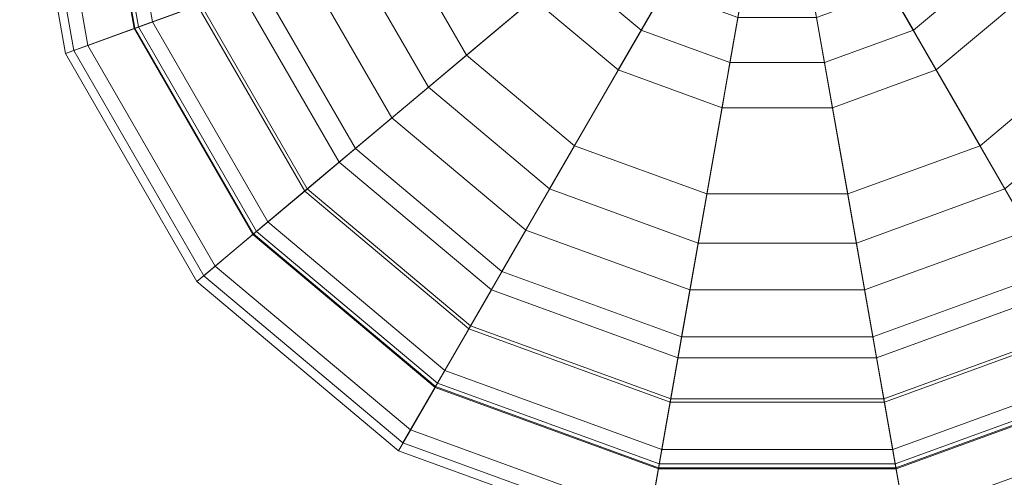
# Model space of a CAD drawing. Units: inches. Extents: x 375 to 1122, y 27 to 1069.
# Tile 41 of 155: x 717.909 to 719.669, y 297.867 to 298.684. Entities that reach past the tile are written whole.
import ezdxf

# ---------------------------------------------------------------- set-up
doc = ezdxf.new("R2010")
doc.units = ezdxf.units.IN
doc.layers.add('Furniture', color=30, linetype='Continuous', lineweight=18)

# ---------------------------------------------------------------- blocks, each defined once
blk = doc.blocks.new('A$C403C54AD')
for points in [[(1.191834, 0.889704, -0.031825), (1.180252, 0.857884, -0.028747), (1.180252, 0.857884, -0.028747), (1.180252, 0.891746, -0.031825)], [(1.202018, 0.883824, -0.031825), (1.180252, 0.857884, -0.028747), (1.180252, 0.857884, -0.028747), (1.191834, 0.889704, -0.031825)], [(1.209578, 0.874815, -0.031825), (1.180252, 0.857884, -0.028747), (1.180252, 0.857884, -0.028747), (1.202018, 0.883824, -0.031825)], [(1.192562, 0.864991, -0.02532), (1.206749, 0.873182, -0.028594), (1.199919, 0.881322, -0.028594), (1.189389, 0.868773, -0.02532)], [(1.193338, 0.873479, 0.061451), (1.186756, 0.865635, 0.054084), (1.183713, 0.867392, 0.054084), (1.187215, 0.877014, 0.061451)], [(1.195951, 0.866948, 0.063639), (1.201568, 0.87019, 0.073031), (1.196073, 0.876739, 0.073031), (1.191904, 0.87177, 0.063639)], [(1.2136, 0.863764, -0.031825), (1.180252, 0.857884, -0.028747), (1.180252, 0.857884, -0.028747), (1.209578, 0.874815, -0.031825)], [(1.185975, 0.864705, 0.057003), (1.191904, 0.87177, 0.063639), (1.186452, 0.874918, 0.063639), (1.183297, 0.866251, 0.057003)], [(1.210344, 0.86319, 0.131159), (1.213207, 0.863695, 0.117935), (1.209232, 0.874616, 0.117935), (1.206714, 0.873162, 0.131159)], [(1.210384, 0.863197, -0.028594), (1.2136, 0.863764, -0.031825), (1.209578, 0.874815, -0.031825), (1.206749, 0.873182, -0.028594)], [(1.213207, 0.863695, 0.117935), (1.212542, 0.863578, 0.089693), (1.208648, 0.874278, 0.089693), (1.209232, 0.874616, 0.117935)], [(1.212542, 0.863578, 0.089693), (1.207259, 0.862646, 0.071684), (1.204002, 0.871596, 0.071684), (1.208648, 0.874278, 0.089693)], [(1.197882, 0.868063, 0.061451), (1.189015, 0.862943, 0.054084), (1.186756, 0.865635, 0.054084), (1.193338, 0.873479, 0.061451)], [(1.19425, 0.860352, -0.02532), (1.210384, 0.863197, -0.028594), (1.206749, 0.873182, -0.028594), (1.192562, 0.864991, -0.02532)], [(1.204491, 0.862158, 0.073031), (1.209521, 0.863045, 0.090178), (1.205991, 0.872744, 0.090178), (1.201568, 0.87019, 0.073031)], [(1.205423, 0.862322, 0.140564), (1.210344, 0.86319, 0.131159), (1.206714, 0.873162, 0.131159), (1.202387, 0.870664, 0.140564)], [(1.210169, 0.863159, 0.117718), (1.207402, 0.862671, 0.130354), (1.204128, 0.871669, 0.130354), (1.206561, 0.873073, 0.117718)], [(1.209521, 0.863045, 0.090178), (1.210169, 0.863159, 0.117718), (1.206561, 0.873073, 0.117718), (1.205991, 0.872744, 0.090178)], [(1.187963, 0.862336, 0.057003), (1.195951, 0.866948, 0.063639), (1.191904, 0.87177, 0.063639), (1.185975, 0.864705, 0.057003)], [(1.207259, 0.862646, 0.071684), (1.2003, 0.861419, 0.061451), (1.197882, 0.868063, 0.061451), (1.204002, 0.871596, 0.071684)], [(1.207402, 0.862671, 0.130354), (1.202392, 0.861788, 0.140564), (1.199721, 0.869125, 0.140564), (1.204128, 0.871669, 0.130354)], [(1.202392, 0.861788, 0.140564), (1.205423, 0.862322, 0.140564), (1.202387, 0.870664, 0.140564), (1.199721, 0.869125, 0.140564)], [(1.198104, 0.861032, 0.063639), (1.204491, 0.862158, 0.073031), (1.201568, 0.87019, 0.073031), (1.195951, 0.866948, 0.063639)], [(1.190789, 0.863967, -0.022455), (1.192562, 0.864991, -0.02532), (1.189389, 0.868773, -0.02532), (1.188073, 0.867204, -0.022455)], [(1.2003, 0.861419, 0.061451), (1.190217, 0.859641, 0.054084), (1.189015, 0.862943, 0.054084), (1.197882, 0.868063, 0.061451)], [(1.187242, 0.861919, -0.020408), (1.190789, 0.863967, -0.022455), (1.188073, 0.867204, -0.022455), (1.18544, 0.864067, -0.020408)], [(1.189021, 0.85943, 0.057003), (1.198104, 0.861032, 0.063639), (1.195951, 0.866948, 0.063639), (1.187963, 0.862336, 0.057003)], [(1.192234, 0.859997, -0.022455), (1.19425, 0.860352, -0.02532), (1.192562, 0.864991, -0.02532), (1.190789, 0.863967, -0.022455)], [(1.1882, 0.859285, -0.020408), (1.192234, 0.859997, -0.022455), (1.190789, 0.863967, -0.022455), (1.187242, 0.861919, -0.020408)], [(1.2136, 0.852004, -0.031825), (1.180252, 0.857884, -0.028747), (1.180252, 0.857884, -0.028747), (1.2136, 0.863764, -0.031825)], [(1.212542, 0.85219, 0.089693), (1.207259, 0.853122, 0.071684), (1.207259, 0.862646, 0.071684), (1.212542, 0.863578, 0.089693)], [(1.210344, 0.852578, 0.131159), (1.213207, 0.852073, 0.117935), (1.213207, 0.863695, 0.117935), (1.210344, 0.86319, 0.131159)], [(1.210384, 0.852571, -0.028594), (1.2136, 0.852004, -0.031825), (1.2136, 0.863764, -0.031825), (1.210384, 0.863197, -0.028594)], [(1.19425, 0.855416, -0.02532), (1.210384, 0.852571, -0.028594), (1.210384, 0.863197, -0.028594), (1.19425, 0.860352, -0.02532)], [(1.205423, 0.853446, 0.140564), (1.210344, 0.852578, 0.131159), (1.210344, 0.86319, 0.131159), (1.205423, 0.862322, 0.140564)], [(1.210169, 0.852609, 0.117718), (1.207402, 0.853097, 0.130354), (1.207402, 0.862671, 0.130354), (1.210169, 0.863159, 0.117718)], [(1.209521, 0.852723, 0.090178), (1.210169, 0.852609, 0.117718), (1.210169, 0.863159, 0.117718), (1.209521, 0.863045, 0.090178)], [(1.207259, 0.853122, 0.071684), (1.2003, 0.854349, 0.061451), (1.2003, 0.861419, 0.061451), (1.207259, 0.862646, 0.071684)], [(1.207402, 0.853097, 0.130354), (1.202392, 0.85398, 0.140564), (1.202392, 0.861788, 0.140564), (1.207402, 0.862671, 0.130354)], [(1.204491, 0.85361, 0.073031), (1.209521, 0.852723, 0.090178), (1.209521, 0.863045, 0.090178), (1.204491, 0.862158, 0.073031)], [(1.202392, 0.85398, 0.140564), (1.205423, 0.853446, 0.140564), (1.205423, 0.862322, 0.140564), (1.202392, 0.861788, 0.140564)], [(1.198104, 0.854736, 0.063639), (1.204491, 0.85361, 0.073031), (1.204491, 0.862158, 0.073031), (1.198104, 0.861032, 0.063639)], [(1.2003, 0.854349, 0.061451), (1.190217, 0.856127, 0.054084), (1.190217, 0.859641, 0.054084), (1.2003, 0.861419, 0.061451)], [(1.189021, 0.856338, 0.057003), (1.198104, 0.854736, 0.063639), (1.198104, 0.861032, 0.063639), (1.189021, 0.85943, 0.057003)], [(1.1882, 0.856482, -0.020408), (1.192234, 0.855771, -0.022455), (1.192234, 0.859997, -0.022455), (1.1882, 0.859285, -0.020408)], [(1.192234, 0.855771, -0.022455), (1.19425, 0.855416, -0.02532), (1.19425, 0.860352, -0.02532), (1.192234, 0.859997, -0.022455)], [(1.209578, 0.840953, -0.031825), (1.180252, 0.857884, -0.028747), (1.180252, 0.857884, -0.028747), (1.2136, 0.852004, -0.031825)], [(1.202018, 0.831944, -0.031825), (1.180252, 0.857884, -0.028747), (1.180252, 0.857884, -0.028747), (1.209578, 0.840953, -0.031825)], [(1.191834, 0.826064, -0.031825), (1.180252, 0.857884, -0.028747), (1.180252, 0.857884, -0.028747), (1.202018, 0.831944, -0.031825)], [(1.180252, 0.824022, -0.031825), (1.180252, 0.857884, -0.028747), (1.180252, 0.857884, -0.028747), (1.191834, 0.826064, -0.031825)], [(1.187242, 0.853848, -0.020408), (1.190789, 0.851801, -0.022455), (1.192234, 0.855771, -0.022455), (1.1882, 0.856482, -0.020408)], [(1.187963, 0.853432, 0.057003), (1.195951, 0.84882, 0.063639), (1.198104, 0.854736, 0.063639), (1.189021, 0.856338, 0.057003)], [(1.197882, 0.847705, 0.061451), (1.189015, 0.852825, 0.054084), (1.190217, 0.856127, 0.054084), (1.2003, 0.854349, 0.061451)], [(1.190789, 0.851801, -0.022455), (1.192562, 0.850777, -0.02532), (1.19425, 0.855416, -0.02532), (1.192234, 0.855771, -0.022455)], [(1.192562, 0.850777, -0.02532), (1.206749, 0.842586, -0.028594), (1.210384, 0.852571, -0.028594), (1.19425, 0.855416, -0.02532)], [(1.195951, 0.84882, 0.063639), (1.201568, 0.845577, 0.073031), (1.204491, 0.85361, 0.073031), (1.198104, 0.854736, 0.063639)], [(1.204002, 0.844172, 0.071684), (1.197882, 0.847705, 0.061451), (1.2003, 0.854349, 0.061451), (1.207259, 0.853122, 0.071684)], [(1.18544, 0.851701, -0.020408), (1.188073, 0.848564, -0.022455), (1.190789, 0.851801, -0.022455), (1.187242, 0.853848, -0.020408)], [(1.199721, 0.846643, 0.140564), (1.202387, 0.845104, 0.140564), (1.205423, 0.853446, 0.140564), (1.202392, 0.85398, 0.140564)], [(1.204128, 0.844099, 0.130354), (1.199721, 0.846643, 0.140564), (1.202392, 0.85398, 0.140564), (1.207402, 0.853097, 0.130354)], [(1.185975, 0.851063, 0.057003), (1.191904, 0.843998, 0.063639), (1.195951, 0.84882, 0.063639), (1.187963, 0.853432, 0.057003)], [(1.201568, 0.845577, 0.073031), (1.205991, 0.843024, 0.090178), (1.209521, 0.852723, 0.090178), (1.204491, 0.85361, 0.073031)], [(1.202387, 0.845104, 0.140564), (1.206714, 0.842606, 0.131159), (1.210344, 0.852578, 0.131159), (1.205423, 0.853446, 0.140564)], [(1.208648, 0.84149, 0.089693), (1.204002, 0.844172, 0.071684), (1.207259, 0.853122, 0.071684), (1.212542, 0.85219, 0.089693)], [(1.206561, 0.842695, 0.117718), (1.204128, 0.844099, 0.130354), (1.207402, 0.853097, 0.130354), (1.210169, 0.852609, 0.117718)], [(1.193338, 0.842289, 0.061451), (1.186756, 0.850133, 0.054084), (1.189015, 0.852825, 0.054084), (1.197882, 0.847705, 0.061451)], [(1.205991, 0.843024, 0.090178), (1.206561, 0.842695, 0.117718), (1.210169, 0.852609, 0.117718), (1.209521, 0.852723, 0.090178)], [(1.206714, 0.842606, 0.131159), (1.209232, 0.841152, 0.117935), (1.213207, 0.852073, 0.117935), (1.210344, 0.852578, 0.131159)], [(1.206749, 0.842586, -0.028594), (1.209578, 0.840953, -0.031825), (1.2136, 0.852004, -0.031825), (1.210384, 0.852571, -0.028594)], [(1.209232, 0.841152, 0.117935), (1.208648, 0.84149, 0.089693), (1.212542, 0.85219, 0.089693), (1.213207, 0.852073, 0.117935)], [(1.188073, 0.848564, -0.022455), (1.189389, 0.846995, -0.02532), (1.192562, 0.850777, -0.02532), (1.190789, 0.851801, -0.022455)], [(1.183297, 0.849517, 0.057003), (1.186452, 0.84085, 0.063639), (1.191904, 0.843998, 0.063639), (1.185975, 0.851063, 0.057003)], [(1.189389, 0.846995, -0.02532), (1.199919, 0.834446, -0.028594), (1.206749, 0.842586, -0.028594), (1.192562, 0.850777, -0.02532)], [(1.187215, 0.838754, 0.061451), (1.183713, 0.848375, 0.054084), (1.186756, 0.850133, 0.054084), (1.193338, 0.842289, 0.061451)], [(1.191904, 0.843998, 0.063639), (1.196073, 0.839029, 0.073031), (1.201568, 0.845577, 0.073031), (1.195951, 0.84882, 0.063639)], [(1.19788, 0.836876, 0.071684), (1.193338, 0.842289, 0.061451), (1.197882, 0.847705, 0.061451), (1.204002, 0.844172, 0.071684)], [(1.185114, 0.844527, -0.02532), (1.190717, 0.829133, -0.028594), (1.199919, 0.834446, -0.028594), (1.189389, 0.846995, -0.02532)], [(1.194703, 0.840662, 0.140564), (1.196681, 0.838304, 0.140564), (1.202387, 0.845104, 0.140564), (1.199721, 0.846643, 0.140564)], [(1.197973, 0.836765, 0.130354), (1.194703, 0.840662, 0.140564), (1.199721, 0.846643, 0.140564), (1.204128, 0.844099, 0.130354)], [(1.196073, 0.839029, 0.073031), (1.199356, 0.835117, 0.090178), (1.205991, 0.843024, 0.090178), (1.201568, 0.845577, 0.073031)], [(1.196681, 0.838304, 0.140564), (1.199893, 0.834477, 0.131159), (1.206714, 0.842606, 0.131159), (1.202387, 0.845104, 0.140564)], [(1.180252, 0.84367, -0.02532), (1.180252, 0.827288, -0.028594), (1.190717, 0.829133, -0.028594), (1.185114, 0.844527, -0.02532)], [(1.201328, 0.832767, 0.089693), (1.19788, 0.836876, 0.071684), (1.204002, 0.844172, 0.071684), (1.208648, 0.84149, 0.089693)], [(1.186452, 0.84085, 0.063639), (1.18867, 0.834755, 0.073031), (1.196073, 0.839029, 0.073031), (1.191904, 0.843998, 0.063639)], [(1.199779, 0.834612, 0.117718), (1.197973, 0.836765, 0.130354), (1.204128, 0.844099, 0.130354), (1.206561, 0.842695, 0.117718)], [(1.199356, 0.835117, 0.090178), (1.199779, 0.834612, 0.117718), (1.206561, 0.842695, 0.117718), (1.205991, 0.843024, 0.090178)], [(1.199893, 0.834477, 0.131159), (1.201762, 0.83225, 0.117935), (1.209232, 0.841152, 0.117935), (1.206714, 0.842606, 0.131159)], [(1.199919, 0.834446, -0.028594), (1.202018, 0.831944, -0.031825), (1.209578, 0.840953, -0.031825), (1.206749, 0.842586, -0.028594)], [(1.189632, 0.832114, 0.071684), (1.187215, 0.838754, 0.061451), (1.193338, 0.842289, 0.061451), (1.19788, 0.836876, 0.071684)], [(1.201762, 0.83225, 0.117935), (1.201328, 0.832767, 0.089693), (1.208648, 0.84149, 0.089693), (1.209232, 0.841152, 0.117935)], [(1.187941, 0.836759, 0.140564), (1.188994, 0.833866, 0.140564), (1.196681, 0.838304, 0.140564), (1.194703, 0.840662, 0.140564)], [(1.189681, 0.831977, 0.130354), (1.187941, 0.836759, 0.140564), (1.194703, 0.840662, 0.140564), (1.197973, 0.836765, 0.130354)], [(1.18867, 0.834755, 0.073031), (1.190417, 0.829956, 0.090178), (1.199356, 0.835117, 0.090178), (1.196073, 0.839029, 0.073031)], [(1.188994, 0.833866, 0.140564), (1.190703, 0.829171, 0.131159), (1.199893, 0.834477, 0.131159), (1.196681, 0.838304, 0.140564)], [(1.191466, 0.827073, 0.089693), (1.189632, 0.832114, 0.071684), (1.19788, 0.836876, 0.071684), (1.201328, 0.832767, 0.089693)], [(1.190642, 0.829337, 0.117718), (1.189681, 0.831977, 0.130354), (1.197973, 0.836765, 0.130354), (1.199779, 0.834612, 0.117718)], [(1.190417, 0.829956, 0.090178), (1.190642, 0.829337, 0.117718), (1.199779, 0.834612, 0.117718), (1.199356, 0.835117, 0.090178)], [(1.180252, 0.833271, 0.073031), (1.180252, 0.828163, 0.090178), (1.190417, 0.829956, 0.090178), (1.18867, 0.834755, 0.073031)], [(1.190703, 0.829171, 0.131159), (1.191697, 0.826439, 0.117935), (1.201762, 0.83225, 0.117935), (1.199893, 0.834477, 0.131159)], [(1.190717, 0.829133, -0.028594), (1.191834, 0.826064, -0.031825), (1.202018, 0.831944, -0.031825), (1.199919, 0.834446, -0.028594)], [(1.180252, 0.832324, 0.140564), (1.180252, 0.827328, 0.131159), (1.190703, 0.829171, 0.131159), (1.188994, 0.833866, 0.140564)], [(1.191697, 0.826439, 0.117935), (1.191466, 0.827073, 0.089693), (1.201328, 0.832767, 0.089693), (1.201762, 0.83225, 0.117935)], [(1.180252, 0.825096, 0.089693), (1.180252, 0.83046, 0.071684), (1.189632, 0.832114, 0.071684), (1.191466, 0.827073, 0.089693)], [(1.180252, 0.827505, 0.117718), (1.180252, 0.830315, 0.130354), (1.189681, 0.831977, 0.130354), (1.190642, 0.829337, 0.117718)], [(1.180252, 0.828163, 0.090178), (1.180252, 0.827505, 0.117718), (1.190642, 0.829337, 0.117718), (1.190417, 0.829956, 0.090178)], [(1.180252, 0.827328, 0.131159), (1.180252, 0.824421, 0.117935), (1.191697, 0.826439, 0.117935), (1.190703, 0.829171, 0.131159)], [(1.180252, 0.827288, -0.028594), (1.180252, 0.824022, -0.031825), (1.191834, 0.826064, -0.031825), (1.190717, 0.829133, -0.028594)], [(1.180252, 0.824421, 0.117935), (1.180252, 0.825096, 0.089693), (1.191466, 0.827073, 0.089693), (1.191697, 0.826439, 0.117935)]]:
    blk.add_3dface(points)

msp = doc.modelspace()

# ---------------------------------------------------------------- block references
at = {"layer": 'Furniture', "xscale": 39.9918517141215, "yscale": 39.9918517141215, "zscale": 39.9918517141215, "rotation": 270}
msp.add_blockref('A$C403C54AD', (684.9549, 346.2875, 0.024), dxfattribs=at)

doc.saveas('drawing.dxf')
